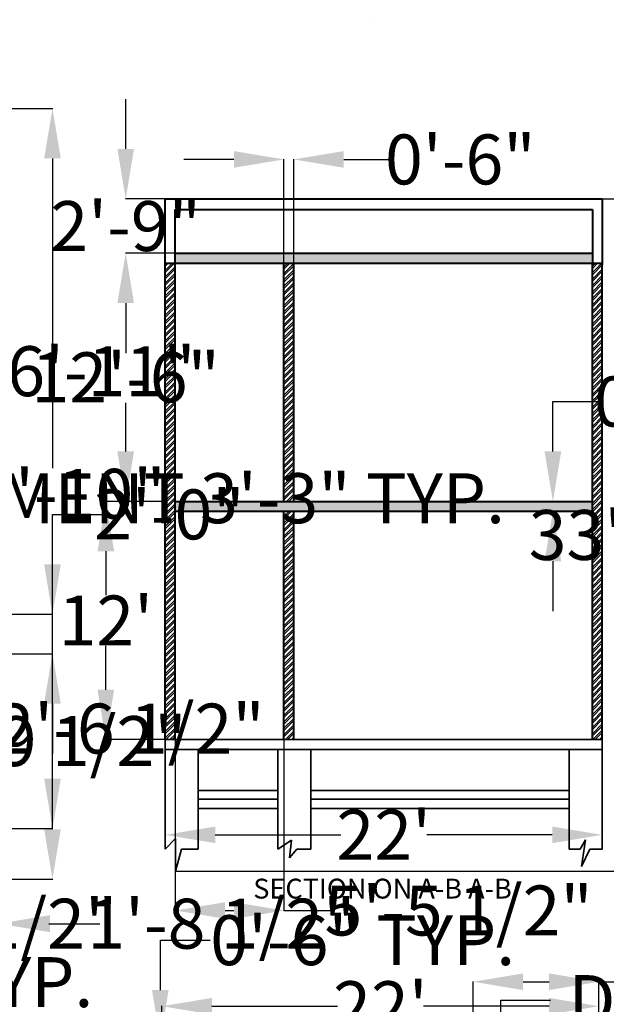
# Model space of a CAD drawing. Units: inches. Extents: x 7323 to 9737, y 2037 to 3322.
# Tile 18 of 19: x 8922 to 9276, y 2709 to 3304. Entities that reach past the tile are written whole.
import ezdxf

# ---------------------------------------------------------------- set-up
doc = ezdxf.new("R2010")
doc.units = ezdxf.units.IN
doc.header["$MEASUREMENT"] = 0
for name, color, linetype, lineweight in [('A-ANNO-DIMS', 2, 'Continuous', 18), ('A-ANNO-TEXT', 7, 'Continuous', 25), ('A-DETL-REFR', 8, 'Continuous', 13), ('A-SECT', 7, 'Continuous', 40), ('S-FNDN', 7, 'Continuous', 35)]:
    doc.layers.add(name, color=color, linetype=linetype, lineweight=lineweight)
doc.layers.add('A-SECT-PATT', color=18, linetype='Continuous', lineweight=13, true_color=0x000000)
doc.layers.add('A-WALL-PATT', color=32, linetype='Continuous', lineweight=13, true_color=0xcd6928)
doc.styles.get("Standard").update_dxf_attribs({"font": 'arial.ttf'})
doc.dimstyles.get("Standard").update_dxf_attribs({"dimtxt": 30.18, "dimasz": 30.18, "dimexe": 0.18, "dimexo": 0.0625, "dimgap": 0.09, "dimtad": 0, "dimtih": 1, "dimtoh": 1, "dimdec": 0, "dimzin": 0, "dimdsep": 46, "dimlunit": 3, "dimtxsty": 'Standard', "dimcen": 0.09, "dimadec": 0, "dimazin": 0, "dimtfac": 1, "dimtdec": 0, "dimtofl": 0, "dimtmove": 0, "dimatfit": 3, "dimfxl": 1, "dimtolj": 1, "dimtzin": 0, "dimarcsym": 0})

# ---------------------------------------------------------------- blocks, each defined once
blk = doc.blocks.new('*D7')
at = {"layer": 'A-ANNO-DIMS', "color": 0, "lineweight": -2, "transparency": 16777216}
for p, q in [((9009.89, 3012.87), (8973.88, 3012.87)), ((8974.06, 2982.69), (8974.06, 2956.11)), ((8974.06, 2899.05), (8974.06, 2925.62)), ((9009.89, 2868.87), (8973.88, 2868.87))]:
    blk.add_line(p, q, dxfattribs=at)
at = {"layer": 'A-ANNO-DIMS', "color": 0, "transparency": 16777216}
for points in [[(8969.03, 2982.69), (8979.09, 2982.69), (8974.06, 3012.87)], [(8969.03, 2899.05), (8979.09, 2899.05), (8974.06, 2868.87)]]:
    blk.add_solid(points, dxfattribs=at)
at = {"layer": 'Defpoints', "color": 0, "transparency": 16777216}
for p in [(8974.06, 3012.87), (9009.95, 3012.87), (9009.95, 2868.87)]:
    blk.add_point(p, dxfattribs=at)
at = {"layer": 'A-ANNO-DIMS', "color": 0, "transparency": 16777216, "insert": (8974.06, 2940.87), "char_height": 30.18, "attachment_point": 5}
blk.add_mtext("\\A1;12'", dxfattribs=at)
blk = doc.blocks.new('*D8')
at = {"layer": 'A-ANNO-DIMS', "color": 0, "lineweight": -2, "transparency": 16777216}
for p, q in [((9009.95, 2862.8), (9009.95, 2811.15)), ((9273.93, 2862.77), (9273.93, 2811.15)), ((9040.13, 2811.33), (9115.98, 2811.33)), ((9243.75, 2811.33), (9167.89, 2811.33))]:
    blk.add_line(p, q, dxfattribs=at)
at = {"layer": 'A-ANNO-DIMS', "color": 0, "transparency": 16777216}
for points in [[(9040.13, 2816.36), (9040.13, 2806.3), (9009.95, 2811.33)], [(9243.75, 2816.36), (9243.75, 2806.3), (9273.93, 2811.33)]]:
    blk.add_solid(points, dxfattribs=at)
at = {"layer": 'Defpoints', "color": 0, "transparency": 16777216}
for p in [(9009.95, 2862.87), (9273.93, 2862.83), (9273.93, 2811.33)]:
    blk.add_point(p, dxfattribs=at)
at = {"layer": 'A-ANNO-DIMS', "color": 0, "transparency": 16777216, "insert": (9141.94, 2811.33), "char_height": 30.18, "attachment_point": 5}
blk.add_mtext("\\A1;22'", dxfattribs=at)
blk = doc.blocks.new('*D10')
at = {"layer": 'A-ANNO-DIMS', "color": 0, "lineweight": -2, "transparency": 16777216}
for p, q in [((9007.95, 2687.36), (9007.95, 2707.94)), ((9038.13, 2707.76), (9113.99, 2707.76)), ((9241.77, 2707.76), (9165.9, 2707.76)), ((9271.95, 2687.36), (9271.95, 2707.94))]:
    blk.add_line(p, q, dxfattribs=at)
at = {"layer": 'A-ANNO-DIMS', "color": 0, "transparency": 16777216}
for points in [[(9038.13, 2712.79), (9038.13, 2702.73), (9007.95, 2707.76)], [(9241.77, 2712.79), (9241.77, 2702.73), (9271.95, 2707.76)]]:
    blk.add_solid(points, dxfattribs=at)
at = {"layer": 'Defpoints', "color": 0, "transparency": 16777216}
for p in [(9271.95, 2707.76), (9007.95, 2687.3), (9271.95, 2687.3)]:
    blk.add_point(p, dxfattribs=at)
at = {"layer": 'A-ANNO-DIMS', "color": 0, "transparency": 16777216, "insert": (9139.95, 2707.76), "char_height": 30.18, "attachment_point": 5}
blk.add_mtext("\\A1;22'", dxfattribs=at)
blk = doc.blocks.new('*D35')
at = {"layer": 'A-ANNO-DIMS', "color": 0, "lineweight": -2, "transparency": 16777216}
for p, q in [((8977.7, 2688.2), (8947.52, 2688.2)), ((9007.88, 2687.36), (9007.88, 2688.38)), ((9013.95, 2687.36), (9013.95, 2688.38)), ((9044.13, 2688.2), (9074.31, 2688.2))]:
    blk.add_line(p, q, dxfattribs=at)
at = {"layer": 'A-ANNO-DIMS', "color": 0, "transparency": 16777216}
for points in [[(8977.7, 2693.23), (8977.7, 2683.17), (9007.88, 2688.2)], [(9044.13, 2693.23), (9044.13, 2683.17), (9013.95, 2688.2)]]:
    blk.add_solid(points, dxfattribs=at)
at = {"layer": 'Defpoints', "color": 0, "transparency": 16777216}
for p in [(9007.88, 2687.3), (9013.95, 2688.2), (9013.95, 2687.3)]:
    blk.add_point(p, dxfattribs=at)
at = {"layer": 'A-ANNO-DIMS', "color": 0, "transparency": 16777216, "insert": (9263.41, 2688.2), "char_height": 30.18, "attachment_point": 5}
blk.add_mtext('\\A1;COLUMN 0\'-6" TYP.', dxfattribs=at)
blk = doc.blocks.new('*D36')
at = {"layer": 'A-ANNO-DIMS', "color": 0, "lineweight": -2, "transparency": 16777216}
for p, q in [((9006.97, 2717.48), (9006.97, 2747.66)), ((9006.97, 2747.66), (9037.15, 2747.66)), ((9007.82, 2687.3), (9006.79, 2687.3)), ((9007.82, 2681.3), (9006.79, 2681.3)), ((9006.97, 2651.12), (9006.97, 2620.94))]:
    blk.add_line(p, q, dxfattribs=at)
at = {"layer": 'A-ANNO-DIMS', "color": 0, "transparency": 16777216}
for points in [[(9001.94, 2717.48), (9012, 2717.48), (9006.97, 2687.3)], [(9001.94, 2651.12), (9012, 2651.12), (9006.97, 2681.3)]]:
    blk.add_solid(points, dxfattribs=at)
at = {"layer": 'Defpoints', "color": 0, "transparency": 16777216}
for p in [(9006.97, 2687.3), (9007.88, 2687.3), (9007.88, 2681.3)]:
    blk.add_point(p, dxfattribs=at)
at = {"layer": 'A-ANNO-DIMS', "color": 0, "transparency": 16777216, "insert": (9129.22, 2747.66), "char_height": 30.18, "attachment_point": 5}
blk.add_mtext('\\A1;0\'-6" TYP.', dxfattribs=at)
blk = doc.blocks.new('*D45')
at = {"layer": 'A-ANNO-DIMS', "color": 0, "lineweight": -2, "transparency": 16777216}
for p, q in [((8725.79, 2664.36), (8695.61, 2664.36)), ((8755.97, 2662.02), (8755.97, 2664.54)), ((8772, 2662.02), (8772, 2664.54)), ((8802.18, 2664.36), (8832.36, 2664.36))]:
    blk.add_line(p, q, dxfattribs=at)
at = {"layer": 'A-ANNO-DIMS', "color": 0, "transparency": 16777216}
for points in [[(8725.79, 2669.39), (8725.79, 2659.33), (8755.97, 2664.36)], [(8802.18, 2669.39), (8802.18, 2659.33), (8772, 2664.36)]]:
    blk.add_solid(points, dxfattribs=at)
at = {"layer": 'Defpoints', "color": 0, "transparency": 16777216}
for p in [(8755.97, 2661.96), (8772, 2664.36), (8772, 2661.96)]:
    blk.add_point(p, dxfattribs=at)
at = {"layer": 'A-ANNO-DIMS', "color": 0, "transparency": 16777216, "insert": (9094.8, 2664.36), "char_height": 30.18, "attachment_point": 5}
blk.add_mtext('\\A1;BEDSIDE TABLE 1\'-4" TYP.', dxfattribs=at)
blk = doc.blocks.new('*D46')
at = {"layer": 'A-ANNO-DIMS', "color": 0, "lineweight": -2, "transparency": 16777216}
for p, q in [((8753.57, 2692.14), (8753.57, 2722.32)), ((8753.57, 2722.32), (8783.75, 2722.32)), ((8755.91, 2661.96), (8753.39, 2661.96)), ((8755.91, 2647.12), (8753.39, 2647.12)), ((8753.57, 2616.94), (8753.57, 2586.76))]:
    blk.add_line(p, q, dxfattribs=at)
at = {"layer": 'A-ANNO-DIMS', "color": 0, "transparency": 16777216}
for points in [[(8748.54, 2692.14), (8758.6, 2692.14), (8753.57, 2661.96)], [(8748.54, 2616.94), (8758.6, 2616.94), (8753.57, 2647.12)]]:
    blk.add_solid(points, dxfattribs=at)
at = {"layer": 'Defpoints', "color": 0, "transparency": 16777216}
for p in [(8753.57, 2661.96), (8755.97, 2661.96), (8755.97, 2647.12)]:
    blk.add_point(p, dxfattribs=at)
at = {"layer": 'A-ANNO-DIMS', "color": 0, "transparency": 16777216, "insert": (8874.4, 2722.32), "char_height": 30.18, "attachment_point": 5}
blk.add_mtext('\\A1;1\'-3" TYP.', dxfattribs=at)
blk = doc.blocks.new('*D57')
at = {"layer": 'A-ANNO-DIMS', "color": 0, "lineweight": -2, "transparency": 16777216}
for p, q in [((8698.34, 3020.54), (8698.34, 3014.6)), ((8737.11, 3020.54), (8737.11, 3014.6)), ((8668.16, 3014.78), (8637.98, 3014.78)), ((8767.29, 3014.78), (8797.47, 3014.78))]:
    blk.add_line(p, q, dxfattribs=at)
at = {"layer": 'A-ANNO-DIMS', "color": 0, "transparency": 16777216}
for points in [[(8668.16, 3019.81), (8668.16, 3009.75), (8698.34, 3014.78)], [(8767.29, 3019.81), (8767.29, 3009.75), (8737.11, 3014.78)]]:
    blk.add_solid(points, dxfattribs=at)
at = {"layer": 'Defpoints', "color": 0, "transparency": 16777216}
for p in [(8698.34, 3020.6), (8737.11, 3020.6), (8737.11, 3014.78)]:
    blk.add_point(p, dxfattribs=at)
at = {"layer": 'A-ANNO-DIMS', "color": 0, "transparency": 16777216, "insert": (9012.35, 3014.78), "char_height": 30.18, "attachment_point": 5}
blk.add_mtext('\\A1;CASEMENT 3\'-3" TYP.', dxfattribs=at)
blk = doc.blocks.new('*D61')
at = {"layer": 'A-ANNO-DIMS', "color": 0, "lineweight": -2, "transparency": 16777216}
for p, q in [((9212.57, 2681.3), (9212.57, 2711.48)), ((9212.57, 2711.48), (9242.75, 2711.48)), ((9201.24, 2681.3), (9212.75, 2681.3)), ((9212.57, 2635.56), (9212.57, 2651.12)), ((9201.24, 2605.38), (9212.75, 2605.38))]:
    blk.add_line(p, q, dxfattribs=at)
at = {"layer": 'A-ANNO-DIMS', "color": 0, "transparency": 16777216}
for points in [[(9207.54, 2651.12), (9217.6, 2651.12), (9212.57, 2681.3)], [(9207.54, 2635.56), (9217.6, 2635.56), (9212.57, 2605.38)]]:
    blk.add_solid(points, dxfattribs=at)
at = {"layer": 'Defpoints', "color": 0, "transparency": 16777216}
for p in [(9201.18, 2681.3), (9212.57, 2681.3), (9201.18, 2605.38)]:
    blk.add_point(p, dxfattribs=at)
at = {"layer": 'A-ANNO-DIMS', "color": 0, "transparency": 16777216, "insert": (9475.82, 2711.48), "char_height": 30.18, "attachment_point": 5}
blk.add_mtext('\\A1;DOUBLE BED 6\'-4" TYP.', dxfattribs=at)
blk = doc.blocks.new('*D83')
at = {"layer": 'A-ANNO-DIMS', "color": 0, "lineweight": -2, "transparency": 16777216}
for p, q in [((8914.96, 3250.33), (8941.98, 3250.33)), ((8941.8, 3220.15), (8941.8, 3032.95)), ((8941.8, 2814.72), (8941.8, 3001.93)), ((8910.13, 2784.54), (8941.98, 2784.54))]:
    blk.add_line(p, q, dxfattribs=at)
at = {"layer": 'A-ANNO-DIMS', "color": 0, "transparency": 16777216}
for points in [[(8936.77, 3220.15), (8946.83, 3220.15), (8941.8, 3250.33)], [(8936.77, 2814.72), (8946.83, 2814.72), (8941.8, 2784.54)]]:
    blk.add_solid(points, dxfattribs=at)
at = {"layer": 'Defpoints', "color": 0, "transparency": 16777216}
for p in [(8914.9, 3250.33), (8941.8, 3250.33), (8910.07, 2784.54)]:
    blk.add_point(p, dxfattribs=at)
at = {"layer": 'A-ANNO-DIMS', "color": 0, "transparency": 16777216, "insert": (8941.8, 3017.44), "char_height": 30.18, "attachment_point": 5}
blk.add_mtext('\\A1;38\'-10"', dxfattribs=at)
blk = doc.blocks.new('*D84')
at = {"layer": 'A-ANNO-DIMS', "color": 0, "lineweight": -2, "transparency": 16777216}
for p, q in [((8778.071366, 2815.126036), (8778.071366, 2757.459848)), ((8910.071366, 2815.126036), (8910.071366, 2757.459848)), ((8747.891366, 2757.639848), (8717.711366, 2757.639848)), ((8940.251366, 2757.639848), (8970.431366, 2757.639848))]:
    blk.add_line(p, q, dxfattribs=at)
at = {"layer": 'A-ANNO-DIMS', "color": 0, "transparency": 16777216}
for points in [[(8747.891366, 2762.669848), (8747.891366, 2752.609848), (8778.071366, 2757.639848)], [(8940.251366, 2762.669848), (8940.251366, 2752.609848), (8910.071366, 2757.639848)]]:
    blk.add_solid(points, dxfattribs=at)
at = {"layer": 'Defpoints', "color": 0, "transparency": 16777216}
for p in [(8778.071366, 2815.188536), (8910.071366, 2815.188536), (8910.071366, 2757.639848)]:
    blk.add_point(p, dxfattribs=at)
at = {"layer": 'A-ANNO-DIMS', "color": 0, "transparency": 16777216, "insert": (8844.071366, 2757.639848), "char_height": 30.18, "attachment_point": 5}
blk.add_mtext('\\A1;11\'-0"', dxfattribs=at)
blk = doc.blocks.new('*D85')
at = {"layer": 'A-ANNO-DIMS', "color": 0, "lineweight": -2, "transparency": 16777216}
for p, q in [((8805.94, 3064.71), (8805.94, 3091.73)), ((8836.12, 3091.55), (8858.99, 3091.55)), ((8889.17, 3064.71), (8889.17, 3091.73)), ((8889.17, 3091.55), (8919.35, 3091.55))]:
    blk.add_line(p, q, dxfattribs=at)
at = {"layer": 'A-ANNO-DIMS', "color": 0, "transparency": 16777216}
for points in [[(8836.12, 3096.58), (8836.12, 3086.52), (8805.94, 3091.55)], [(8858.99, 3096.58), (8858.99, 3086.52), (8889.17, 3091.55)]]:
    blk.add_solid(points, dxfattribs=at)
at = {"layer": 'Defpoints', "color": 0, "transparency": 16777216}
for p in [(8889.17, 3091.55), (8805.94, 3064.65), (8889.17, 3064.65)]:
    blk.add_point(p, dxfattribs=at)
at = {"layer": 'A-ANNO-DIMS', "color": 0, "transparency": 16777216, "insert": (8971.36, 3091.55), "char_height": 30.18, "attachment_point": 5}
blk.add_mtext('\\A1;6\'-11"', dxfattribs=at)
blk = doc.blocks.new('*D88')
at = {"layer": 'A-ANNO-DIMS', "color": 0, "lineweight": -2, "transparency": 16777216}
for p, q in [((8941.797746, 2974.828285), (8941.797746, 3005.008285)), ((8941.797746, 3005.008285), (8971.977746, 3005.008285)), ((8847.615005, 2944.648285), (8941.977746, 2944.648285)), ((8909.54808, 2920.815964), (8941.977746, 2920.815964)), ((8941.797746, 2890.635964), (8941.797746, 2860.455964))]:
    blk.add_line(p, q, dxfattribs=at)
at = {"layer": 'A-ANNO-DIMS', "color": 0, "transparency": 16777216}
for points in [[(8936.767746, 2974.828285), (8946.827746, 2974.828285), (8941.797746, 2944.648285)], [(8936.767746, 2890.635964), (8946.827746, 2890.635964), (8941.797746, 2920.815964)]]:
    blk.add_solid(points, dxfattribs=at)
at = {"layer": 'Defpoints', "color": 0, "transparency": 16777216}
for p in [(8847.552505, 2944.648285), (8941.797746, 2944.648285), (8909.48558, 2920.815964)]:
    blk.add_point(p, dxfattribs=at)
at = {"layer": 'A-ANNO-DIMS', "color": 0, "transparency": 16777216, "insert": (9012.438128, 3005.008285), "char_height": 30.18, "attachment_point": 5}
blk.add_mtext('\\A1;2\'-0"', dxfattribs=at)
blk = doc.blocks.new('*D90')
at = {"layer": 'A-ANNO-DIMS', "color": 0, "lineweight": -2, "transparency": 16777216}
for p, q in [((8718.91, 2815.13), (8718.91, 2757.46)), ((8764.24, 2815.13), (8764.24, 2757.46)), ((8688.73, 2757.64), (8658.55, 2757.64)), ((8794.42, 2757.64), (8824.6, 2757.64))]:
    blk.add_line(p, q, dxfattribs=at)
at = {"layer": 'A-ANNO-DIMS', "color": 0, "transparency": 16777216}
for points in [[(8688.73, 2762.67), (8688.73, 2752.61), (8718.91, 2757.64)], [(8794.42, 2762.67), (8794.42, 2752.61), (8764.24, 2757.64)]]:
    blk.add_solid(points, dxfattribs=at)
at = {"layer": 'Defpoints', "color": 0, "transparency": 16777216}
for p in [(8718.91, 2815.19), (8764.24, 2815.19), (8764.24, 2757.64)]:
    blk.add_point(p, dxfattribs=at)
at = {"layer": 'A-ANNO-DIMS', "color": 0, "transparency": 16777216, "insert": (8899.95, 2757.64), "char_height": 30.18, "attachment_point": 5}
blk.add_mtext('\\A1;3\'-9 1/2"', dxfattribs=at)
blk = doc.blocks.new('*D91')
at = {"layer": 'A-ANNO-DIMS', "color": 0, "lineweight": -2, "transparency": 16777216}
for p, q in [((8909.55, 2920.82), (8941.98, 2920.82)), ((8941.8, 2890.64), (8941.8, 2883.7)), ((8941.8, 2845.37), (8941.8, 2852.31)), ((8910.13, 2815.19), (8941.98, 2815.19))]:
    blk.add_line(p, q, dxfattribs=at)
at = {"layer": 'A-ANNO-DIMS', "color": 0, "transparency": 16777216}
for points in [[(8936.77, 2890.64), (8946.83, 2890.64), (8941.8, 2920.82)], [(8936.77, 2845.37), (8946.83, 2845.37), (8941.8, 2815.19)]]:
    blk.add_solid(points, dxfattribs=at)
at = {"layer": 'Defpoints', "color": 0, "transparency": 16777216}
for p in [(8909.49, 2920.82), (8941.8, 2920.82), (8910.07, 2815.19)]:
    blk.add_point(p, dxfattribs=at)
at = {"layer": 'A-ANNO-DIMS', "color": 0, "transparency": 16777216, "insert": (8941.8, 2868), "char_height": 30.18, "attachment_point": 5}
blk.add_mtext('\\A1;8\'-9 1/2"', dxfattribs=at)
blk = doc.blocks.new('*D92')
at = {"layer": 'A-ANNO-DIMS', "color": 0, "lineweight": -2, "transparency": 16777216}
for p, q in [((8883.17, 2845.37), (8883.17, 2875.55)), ((8883.17, 2875.55), (8913.35, 2875.55)), ((8910.01, 2815.19), (8882.99, 2815.19)), ((8910.01, 2784.54), (8882.99, 2784.54)), ((8883.17, 2754.36), (8883.17, 2724.18))]:
    blk.add_line(p, q, dxfattribs=at)
at = {"layer": 'A-ANNO-DIMS', "color": 0, "transparency": 16777216}
for points in [[(8878.14, 2845.37), (8888.2, 2845.37), (8883.17, 2815.19)], [(8878.14, 2754.36), (8888.2, 2754.36), (8883.17, 2784.54)]]:
    blk.add_solid(points, dxfattribs=at)
at = {"layer": 'Defpoints', "color": 0, "transparency": 16777216}
for p in [(8883.17, 2815.19), (8910.07, 2815.19), (8910.07, 2784.54)]:
    blk.add_point(p, dxfattribs=at)
at = {"layer": 'A-ANNO-DIMS', "color": 0, "transparency": 16777216, "insert": (8988.97, 2875.55), "char_height": 30.18, "attachment_point": 5}
blk.add_mtext('\\A1;2\'-6 1/2"', dxfattribs=at)
blk = doc.blocks.new('*D93')
at = {"layer": 'A-ANNO-DIMS', "color": 0, "lineweight": -2, "transparency": 16777216}
for p, q in [((9274.01, 3195.71), (9297.98, 3195.71)), ((9297.8, 3165.53), (9297.8, 3008.09)), ((9297.8, 2819.64), (9297.8, 2977.07)), ((9016.27, 2789.46), (9297.98, 2789.46))]:
    blk.add_line(p, q, dxfattribs=at)
at = {"layer": 'A-ANNO-DIMS', "color": 0, "transparency": 16777216}
for points in [[(9292.77, 3165.53), (9302.83, 3165.53), (9297.8, 3195.71)], [(9292.77, 2819.64), (9302.83, 2819.64), (9297.8, 2789.46)]]:
    blk.add_solid(points, dxfattribs=at)
at = {"layer": 'Defpoints', "color": 0, "transparency": 16777216}
for p in [(9273.95, 3195.71), (9297.8, 3195.71), (9016.21, 2789.46)]:
    blk.add_point(p, dxfattribs=at)
at = {"layer": 'A-ANNO-DIMS', "color": 0, "transparency": 16777216, "insert": (9297.8, 2992.58), "char_height": 30.18, "attachment_point": 5}
blk.add_mtext('\\A1;33\'-10"', dxfattribs=at)
blk = doc.blocks.new('*D94')
at = {"layer": 'A-ANNO-DIMS', "color": 0, "lineweight": -2, "transparency": 16777216}
for p, q in [((9015.89, 3162.87), (8985.86, 3162.87)), ((8986.04, 3132.69), (8986.04, 3103.37)), ((8986.04, 3043.05), (8986.04, 3072.37)), ((9009.89, 3012.87), (8985.86, 3012.87))]:
    blk.add_line(p, q, dxfattribs=at)
at = {"layer": 'A-ANNO-DIMS', "color": 0, "transparency": 16777216}
for points in [[(8981.01, 3132.69), (8991.07, 3132.69), (8986.04, 3162.87)], [(8981.01, 3043.05), (8991.07, 3043.05), (8986.04, 3012.87)]]:
    blk.add_solid(points, dxfattribs=at)
at = {"layer": 'Defpoints', "color": 0, "transparency": 16777216}
for p in [(8986.04, 3162.87), (9015.95, 3162.87), (9009.95, 3012.87)]:
    blk.add_point(p, dxfattribs=at)
at = {"layer": 'A-ANNO-DIMS', "color": 0, "transparency": 16777216, "insert": (8986.04, 3087.87), "char_height": 30.18, "attachment_point": 5}
blk.add_mtext('\\A1;12\'-6"', dxfattribs=at)
blk = doc.blocks.new('*D95')
at = {"layer": 'A-ANNO-DIMS', "color": 0, "lineweight": -2, "transparency": 16777216}
for p, q in [((9015.95, 2868.8), (9015.95, 2765.43)), ((9081.6, 2868.8), (9081.6, 2765.43)), ((9046.13, 2765.61), (9051.42, 2765.61)), ((9081.6, 2765.61), (9111.78, 2765.61))]:
    blk.add_line(p, q, dxfattribs=at)
at = {"layer": 'A-ANNO-DIMS', "color": 0, "transparency": 16777216}
for points in [[(9046.13, 2770.64), (9046.13, 2760.58), (9015.95, 2765.61)], [(9051.42, 2770.64), (9051.42, 2760.58), (9081.6, 2765.61)]]:
    blk.add_solid(points, dxfattribs=at)
at = {"layer": 'Defpoints', "color": 0, "transparency": 16777216}
for p in [(9015.95, 2868.87), (9081.6, 2868.87), (9081.6, 2765.61)]:
    blk.add_point(p, dxfattribs=at)
at = {"layer": 'A-ANNO-DIMS', "color": 0, "transparency": 16777216, "insert": (9187.14, 2765.61), "char_height": 30.18, "attachment_point": 5}
blk.add_mtext('\\A1;5\'-5 1/2"', dxfattribs=at)
blk = doc.blocks.new('*D96')
at = {"layer": 'A-ANNO-DIMS', "color": 0, "lineweight": -2, "transparency": 16777216}
for p, q in [((8986.035629, 3225.888167), (8986.035629, 3256.068167)), ((9009.885629, 3195.708167), (8985.855629, 3195.708167)), ((9015.885629, 3162.866511), (8985.855629, 3162.866511)), ((8986.035629, 3132.686511), (8986.035629, 3102.506511))]:
    blk.add_line(p, q, dxfattribs=at)
at = {"layer": 'A-ANNO-DIMS', "color": 0, "transparency": 16777216}
for points in [[(8981.005629, 3225.888167), (8991.065629, 3225.888167), (8986.035629, 3195.708167)], [(8981.005629, 3132.686511), (8991.065629, 3132.686511), (8986.035629, 3162.866511)]]:
    blk.add_solid(points, dxfattribs=at)
at = {"layer": 'Defpoints', "color": 0, "transparency": 16777216}
for p in [(8986.035629, 3195.708167), (9009.948129, 3195.708167), (9015.948129, 3162.866511)]:
    blk.add_point(p, dxfattribs=at)
at = {"layer": 'A-ANNO-DIMS', "color": 0, "transparency": 16777216, "insert": (8986.035629, 3179.287339), "char_height": 30.18, "attachment_point": 5}
blk.add_mtext('\\A1;2\'-9"', dxfattribs=at)
blk = doc.blocks.new('*D101')
at = {"layer": 'A-ANNO-DIMS', "color": 0, "lineweight": -2, "transparency": 16777216}
for p, q in [((8889.17, 2984.59), (8889.17, 2757.46)), ((8909.49, 2920.75), (8909.49, 2757.46)), ((8858.99, 2757.64), (8828.81, 2757.64)), ((8939.67, 2757.64), (8969.85, 2757.64))]:
    blk.add_line(p, q, dxfattribs=at)
at = {"layer": 'A-ANNO-DIMS', "color": 0, "transparency": 16777216}
for points in [[(8858.99, 2762.67), (8858.99, 2752.61), (8889.17, 2757.64)], [(8939.67, 2762.67), (8939.67, 2752.61), (8909.49, 2757.64)]]:
    blk.add_solid(points, dxfattribs=at)
at = {"layer": 'Defpoints', "color": 0, "transparency": 16777216}
for p in [(8889.17, 2984.65), (8909.49, 2920.82), (8909.49, 2757.64)]:
    blk.add_point(p, dxfattribs=at)
at = {"layer": 'A-ANNO-DIMS', "color": 0, "transparency": 16777216, "insert": (9043.79, 2757.64), "char_height": 30.18, "attachment_point": 5}
blk.add_mtext('\\A1;1\'-8 1/2"', dxfattribs=at)
blk = doc.blocks.new('*D103')
at = {"layer": 'A-ANNO-DIMS', "color": 0, "lineweight": -2, "transparency": 16777216}
for p, q in [((9244.1, 3043.05), (9244.1, 3073.23)), ((9244.1, 3073.23), (9274.28, 3073.23)), ((9267.89, 3012.87), (9243.92, 3012.87)), ((9267.89, 3006.87), (9243.92, 3006.87)), ((9244.1, 2976.69), (9244.1, 2946.51))]:
    blk.add_line(p, q, dxfattribs=at)
at = {"layer": 'A-ANNO-DIMS', "color": 0, "transparency": 16777216}
for points in [[(9239.07, 3043.05), (9249.13, 3043.05), (9244.1, 3012.87)], [(9239.07, 2976.69), (9249.13, 2976.69), (9244.1, 3006.87)]]:
    blk.add_solid(points, dxfattribs=at)
at = {"layer": 'Defpoints', "color": 0, "transparency": 16777216}
for p in [(9244.1, 3012.87), (9267.95, 3012.87), (9267.95, 3006.87)]:
    blk.add_point(p, dxfattribs=at)
at = {"layer": 'A-ANNO-DIMS', "color": 0, "transparency": 16777216, "insert": (9314.48, 3073.23), "char_height": 30.18, "attachment_point": 5}
blk.add_mtext('\\A1;0\'-6"', dxfattribs=at)
blk = doc.blocks.new('*D104')
at = {"layer": 'A-ANNO-DIMS', "color": 0, "lineweight": -2, "transparency": 16777216}
for p, q in [((9051.42, 3219.56), (9021.24, 3219.56)), ((9081.6, 3156.93), (9081.6, 3219.74)), ((9087.6, 3156.93), (9087.6, 3219.74)), ((9117.78, 3219.56), (9147.96, 3219.56))]:
    blk.add_line(p, q, dxfattribs=at)
at = {"layer": 'A-ANNO-DIMS', "color": 0, "transparency": 16777216}
for points in [[(9051.42, 3224.59), (9051.42, 3214.53), (9081.6, 3219.56)], [(9117.78, 3224.59), (9117.78, 3214.53), (9087.6, 3219.56)]]:
    blk.add_solid(points, dxfattribs=at)
at = {"layer": 'Defpoints', "color": 0, "transparency": 16777216}
for p in [(9087.6, 3219.56), (9081.6, 3156.87), (9087.6, 3156.87)]:
    blk.add_point(p, dxfattribs=at)
at = {"layer": 'A-ANNO-DIMS', "color": 0, "transparency": 16777216, "insert": (9188.16, 3219.56), "char_height": 30.18, "attachment_point": 5}
blk.add_mtext('\\A1;0\'-6"', dxfattribs=at)
blk = doc.blocks.new('*D123')
at = {"layer": 'A-ANNO-DIMS', "color": 0, "lineweight": -2, "transparency": 16777216}
for p, q in [((9195.95, 2687.36), (9195.95, 2722.73)), ((9226.13, 2722.55), (9241.77, 2722.55)), ((9271.95, 2687.36), (9271.95, 2722.73)), ((9271.95, 2722.55), (9302.13, 2722.55))]:
    blk.add_line(p, q, dxfattribs=at)
at = {"layer": 'A-ANNO-DIMS', "color": 0, "transparency": 16777216}
for points in [[(9226.13, 2727.58), (9226.13, 2717.52), (9195.95, 2722.55)], [(9241.77, 2727.58), (9241.77, 2717.52), (9271.95, 2722.55)]]:
    blk.add_solid(points, dxfattribs=at)
at = {"layer": 'Defpoints', "color": 0, "transparency": 16777216}
for p in [(9271.95, 2722.55), (9195.95, 2687.3), (9271.95, 2687.3)]:
    blk.add_point(p, dxfattribs=at)
at = {"layer": 'A-ANNO-DIMS', "color": 0, "transparency": 16777216, "insert": (9342.41, 2722.55), "char_height": 30.18, "attachment_point": 5}
blk.add_mtext('\\A1;6\'-4"', dxfattribs=at)

msp = doc.modelspace()

# ---------------------------------------------------------------- hatches: boundary and pattern name
at = {"layer": 'A-SECT-PATT'}
h = msp.add_hatch(color=256, dxfattribs=at)
h.dxf.hatch_style = 1
h.paths.add_polyline_path([(9267.95, 3162.87), (9139.95, 3162.87), (9015.95, 3162.87), (9015.95, 3156.87), (9139.95, 3156.87), (9141.95, 3156.87), (9267.95, 3156.87)])
h.paths.add_polyline_path([(9267.95, 3012.87), (9141.95, 3012.87), (9087.6, 3012.87), (9087.6, 3006.87), (9141.95, 3006.87), (9267.95, 3006.87)])
h.paths.add_polyline_path([(9081.6, 3012.87), (9015.95, 3012.87), (9015.95, 3006.87), (9081.6, 3006.87)])
h = msp.add_hatch(color=256, dxfattribs=at)
h.dxf.hatch_style = 1
h.paths.add_polyline_path([(9267.95, 3012.87), (9141.95, 3012.87), (9087.6, 3012.87), (9081.6, 3012.87), (9015.95, 3012.87), (9015.95, 3006.87), (9081.6, 3006.87), (9087.6, 3006.87), (9141.95, 3006.87), (9267.95, 3006.87)])
at = {"layer": 'A-WALL-PATT'}
h = msp.add_hatch(dxfattribs=at)
h.set_pattern_fill('ANSI32', color=256, scale=7.3)
h.paths.add_polyline_path([(9273.95, 3156.87), (9267.95, 3156.87), (9267.95, 2868.87), (9273.95, 2868.87)])
h.paths.add_polyline_path([(9015.95, 3156.87), (9011.95, 3156.87), (9009.95, 3156.87), (9009.95, 3012.87), (9009.95, 2868.87), (9015.95, 2868.87), (9015.95, 3012.87)])
h.paths.add_polyline_path([(9081.6, 3012.87), (9087.6, 3012.87), (9087.6, 3156.87), (9081.6, 3156.87)])
h.paths.add_polyline_path([(9087.6, 3006.87), (9081.6, 3006.87), (9081.6, 2868.87), (9087.6, 2868.87)])

# ---------------------------------------------------------------- linework, layer by layer
at = {"layer": 'A-DETL-REFR'}
msp.add_lwpolyline([(9135.51, 3304.01), (9135.51, 3304.01)], close=True, dxfattribs=at)
at = {"layer": 'A-SECT'}
for p, q in [((9009.95, 3156.87), (9009.95, 3195.71)), ((9009.95, 3195.71), (9273.95, 3195.71)), ((9273.95, 3195.71), (9273.95, 3155.83)), ((9015.95, 3156.87), (9015.95, 3189.22)), ((9015.95, 3189.22), (9267.95, 3189.22)), ((9267.95, 3189.22), (9267.95, 3162.87)), ((9139.95, 3162.87), (9267.95, 3162.87)), ((9267.95, 3162.87), (9267.95, 3156.87)), ((9009.95, 3012.87), (9009.95, 3156.87)), ((9009.95, 3156.87), (9141.95, 3156.87)), ((9015.95, 3012.87), (9015.95, 3156.87)), ((9081.6, 3012.87), (9081.6, 3156.87)), ((9087.6, 3012.87), (9087.6, 3156.87)), ((9139.95, 3156.87), (9273.95, 3156.87)), ((9267.95, 2868.87), (9267.95, 3156.87)), ((9273.95, 2868.87), (9273.95, 3156.87)), ((9009.95, 2868.87), (9009.95, 3012.87)), ((9015.95, 3012.87), (9081.6, 3012.87)), ((9015.95, 2868.87), (9015.95, 3012.87)), ((9081.6, 3012.87), (9087.6, 3012.87)), ((9087.6, 3012.87), (9141.95, 3012.87)), ((9141.95, 3012.87), (9267.95, 3012.87)), ((9015.95, 3006.87), (9081.6, 3006.87)), ((9081.6, 2868.87), (9081.6, 3006.87)), ((9081.6, 3006.87), (9087.6, 3006.87)), ((9087.6, 2868.87), (9087.6, 3006.87)), ((9087.6, 3006.87), (9141.95, 3006.87)), ((9141.95, 3006.87), (9267.95, 3006.87))]:
    msp.add_line(p, q, dxfattribs=at)
for points in [[(9015.95, 3162.87), (9139.95, 3162.87)], [(9011.95, 3156.87), (9139.95, 3156.87)]]:
    msp.add_lwpolyline(points, dxfattribs=at)
at = {"layer": 'S-FNDN'}
for p, q in [((9273.95, 2868.87), (9009.95, 2868.87)), ((9009.95, 2868.87), (9009.95, 2838.22)), ((9273.95, 2838.22), (9273.95, 2868.87)), ((9273.95, 2862.87), (9009.95, 2862.87)), ((9009.95, 2862.87), (9273.95, 2862.87)), ((9029.78, 2838.22), (9077.88, 2838.22)), ((9029.78, 2832.82), (9077.88, 2832.82)), ((9097.78, 2838.22), (9254.03, 2838.22)), ((9097.78, 2832.82), (9254.03, 2832.82)), ((9273.93, 2838.22), (9273.95, 2838.22)), ((9029.78, 2827.3), (9077.88, 2827.3)), ((9097.78, 2827.3), (9254.03, 2827.3)), ((9009.89, 2802.77), (9016.21, 2809.1)), ((9016.21, 2809.1), (9016.21, 2789.46)), ((9077.88, 2802.77), (9086.16, 2808.15)), ((9086.16, 2808.15), (9084.96, 2797.42)), ((9260.49, 2802.77), (9263.7, 2808.32)), ((9263.7, 2808.32), (9261.4, 2792.22)), ((9016.21, 2789.46), (9019.83, 2802.77)), ((9084.96, 2797.42), (9089.37, 2802.77)), ((9254.03, 2802.77), (9260.49, 2802.77)), ((9261.4, 2792.22), (9266.34, 2802.77))]:
    msp.add_line(p, q, dxfattribs=at)
for points in [[(9009.89, 2802.77), (9009.89, 2802.77), (9009.89, 2868.87), (9009.89, 2868.87), (9029.78, 2868.87), (9029.78, 2868.87)], [(9077.88, 2868.87), (9077.88, 2868.87), (9097.78, 2868.87), (9097.78, 2868.87)], [(9029.78, 2862.87), (9029.78, 2802.77), (9029.78, 2802.77), (9019.83, 2802.77)], [(9077.88, 2802.77), (9077.88, 2802.77), (9077.88, 2862.87)], [(9097.78, 2862.87), (9097.78, 2802.77), (9097.78, 2802.77), (9089.37, 2802.77)], [(9260.49, 2802.77), (9254.03, 2802.77), (9254.03, 2802.77), (9254.03, 2862.87)], [(9273.93, 2862.87), (9273.93, 2802.77), (9273.93, 2802.77), (9266.34, 2802.77)]]:
    msp.add_lwpolyline(points, dxfattribs=at)

# ---------------------------------------------------------------- texts
at = {"layer": 'A-ANNO-TEXT', "insert": (9063.1, 2784.84), "char_height": 12, "attachment_point": 1}
msp.add_mtext_dynamic_manual_height_columns('SECTION ON A-B A-B', width=349.8601, gutter_width=1, heights=[0], dxfattribs=at)

# ---------------------------------------------------------------- dimensions: what is measured, and where the dimension line sits
at = {"layer": 'A-ANNO-DIMS'}
for base, p1, p2, override, picture, middle in [((8986.04, 3195.71), (9015.95, 3162.87), (9009.95, 3195.71), {"dimdec": 1, "dimlfac": 1, "dimrnd": 0, "dimzin": 1, "dimdsep": 46, "dimlunit": 4, "dimfrac": 2}, '*D96', (8986.04, 3179.29)), ((8941.8, 3250.33), (8910.07, 2784.54), (8914.9, 3250.33), {"dimdec": 1, "dimlfac": 1, "dimrnd": 0, "dimzin": 1, "dimdsep": 46, "dimlunit": 4, "dimfrac": 2}, '*D83', (8941.8, 3017.44)), ((9297.7981, 3195.7082), (9016.212, 2789.4588), (9273.9481, 3195.7082), {"dimdec": 1, "dimlfac": 1, "dimrnd": 0, "dimzin": 1, "dimdsep": 46, "dimlunit": 4, "dimfrac": 2}, '*D93', (9297.7981, 2992.5835)), ((8986.04, 3162.87), (9009.95, 3012.87), (9015.95, 3162.87), {"dimdec": 1, "dimlfac": 1, "dimrnd": 0, "dimzin": 1, "dimdsep": 46, "dimlunit": 4, "dimfrac": 2}, '*D94', (8986.04, 3087.87)), ((9244.1, 3012.87), (9267.95, 3006.87), (9267.95, 3012.87), {"dimdec": 1, "dimlfac": 1, "dimrnd": 0, "dimzin": 1, "dimdsep": 46, "dimlunit": 4, "dimfrac": 2}, '*D103', (9314.48, 3073.23)), ((8941.8, 2944.65), (8909.49, 2920.82), (8847.55, 2944.65), {"dimdec": 1, "dimlfac": 1, "dimrnd": 0, "dimzin": 1, "dimdsep": 46, "dimlunit": 4, "dimfrac": 2}, '*D88', (9012.44, 3005.01)), ((8974.06, 3012.87), (9009.95, 2868.87), (9009.95, 3012.87), {"dimclrd": 0, "dimclre": 0, "dimclrt": 0}, '*D7', (8974.06, 2940.87)), ((8941.8, 2920.82), (8910.07, 2815.19), (8909.49, 2920.82), {"dimdec": 1, "dimlfac": 1, "dimrnd": 0, "dimzin": 1, "dimdsep": 46, "dimlunit": 4, "dimfrac": 2}, '*D91', (8941.8, 2868)), ((8883.1714, 2815.1885), (8910.0714, 2784.5398), (8910.0714, 2815.1885), {"dimdec": 1, "dimlfac": 1, "dimrnd": 0, "dimzin": 1, "dimdsep": 46, "dimlunit": 4, "dimfrac": 2}, '*D92', (8988.9737, 2875.5485))]:
    dim = msp.add_linear_dim(base=base, p1=p1, p2=p2, angle=90, dimstyle='Standard', override=override, dxfattribs=at)
    dim.commit()
    dim.dimension.update_dxf_attribs({"geometry": picture, "text_midpoint": middle})
for base, p1, p2, override, picture, middle in [((9087.6, 3219.56), (9081.6, 3156.87), (9087.6, 3156.87), {"dimdec": 1, "dimlfac": 1, "dimrnd": 0, "dimzin": 1, "dimdsep": 46, "dimlunit": 4, "dimfrac": 2}, '*D104', (9188.16, 3219.56)), ((8889.17, 3091.55), (8805.94, 3064.65), (8889.17, 3064.65), {"dimdec": 1, "dimlfac": 1, "dimrnd": 0, "dimzin": 1, "dimdsep": 46, "dimlunit": 4, "dimfrac": 2}, '*D85', (8971.36, 3091.55)), ((8909.49, 2757.64), (8889.17, 2984.65), (8909.49, 2920.82), {"dimdec": 1, "dimlfac": 1, "dimrnd": 0, "dimzin": 1, "dimdsep": 46, "dimlunit": 4, "dimfrac": 2}, '*D101', (9043.79, 2757.64)), ((9081.5953, 2765.6088), (9015.9481, 2868.8665), (9081.5953, 2868.8665), {"dimdec": 1, "dimlfac": 1, "dimrnd": 0, "dimzin": 1, "dimdsep": 46, "dimlunit": 4, "dimfrac": 2}, '*D95', (9187.1403, 2765.6088)), ((9273.93, 2811.33), (9009.95, 2862.87), (9273.93, 2862.83), {"dimclrd": 0, "dimclre": 0, "dimclrt": 0}, '*D8', (9141.94, 2811.33)), ((8764.24, 2757.64), (8718.91, 2815.19), (8764.24, 2815.19), {"dimdec": 1, "dimlfac": 1, "dimrnd": 0, "dimzin": 1, "dimdsep": 46, "dimlunit": 4, "dimfrac": 2}, '*D90', (8899.95, 2757.64)), ((8910.07, 2757.64), (8778.07, 2815.19), (8910.07, 2815.19), {"dimdec": 1, "dimlfac": 1, "dimrnd": 0, "dimzin": 1, "dimdsep": 46, "dimlunit": 4, "dimfrac": 2}, '*D84', (8844.07, 2757.64)), ((9271.95, 2722.55), (9195.95, 2687.3), (9271.95, 2687.3), {"dimdec": 1, "dimlfac": 1, "dimrnd": 0, "dimzin": 1, "dimdsep": 46, "dimlunit": 4, "dimfrac": 2}, '*D123', (9342.41, 2722.55)), ((9271.95, 2707.76), (9007.95, 2687.3), (9271.95, 2687.3), {"dimclrd": 0, "dimclre": 0, "dimclrt": 0}, '*D10', (9139.95, 2707.76))]:
    dim = msp.add_linear_dim(base=base, p1=p1, p2=p2, dimstyle='Standard', override=override, dxfattribs=at)
    dim.commit()
    dim.dimension.update_dxf_attribs({"geometry": picture, "text_midpoint": middle})
for base, p1, p2, text, picture, middle in [((8737.11, 3014.78), (8698.34, 3020.6), (8737.11, 3020.6), 'CASEMENT <> TYP.', '*D57', (9012.35, 3014.78)), ((8772, 2664.36), (8755.97, 2661.96), (8772, 2661.96), 'BEDSIDE TABLE <> TYP.', '*D45', (9094.8, 2664.36)), ((9013.95, 2688.2), (9007.88, 2687.3), (9013.95, 2687.3), 'COLUMN <> TYP.', '*D35', (9263.41, 2688.2))]:
    dim = msp.add_linear_dim(base=base, p1=p1, p2=p2, text=text, dimstyle='Standard', override={"dimdec": 1, "dimlfac": 1, "dimrnd": 0, "dimzin": 1, "dimdsep": 46, "dimlunit": 4, "dimfrac": 2}, dxfattribs=at)
    dim.commit()
    dim.dimension.update_dxf_attribs({"geometry": picture, "text_midpoint": middle})
for base, p1, p2, text, picture, middle in [((9212.57, 2681.3), (9201.18, 2605.38), (9201.18, 2681.3), 'DOUBLE BED <> TYP.', '*D61', (9475.82, 2711.48)), ((9006.97, 2687.3), (9007.88, 2681.3), (9007.88, 2687.3), '<> TYP.', '*D36', (9129.22, 2747.66)), ((8753.57, 2661.96), (8755.97, 2647.12), (8755.97, 2661.96), '<> TYP.', '*D46', (8874.4, 2722.32))]:
    dim = msp.add_linear_dim(base=base, p1=p1, p2=p2, angle=90, text=text, dimstyle='Standard', override={"dimdec": 1, "dimlfac": 1, "dimrnd": 0, "dimzin": 1, "dimdsep": 46, "dimlunit": 4, "dimfrac": 2}, dxfattribs=at)
    dim.commit()
    dim.dimension.update_dxf_attribs({"geometry": picture, "text_midpoint": middle})

doc.saveas('drawing.dxf')
